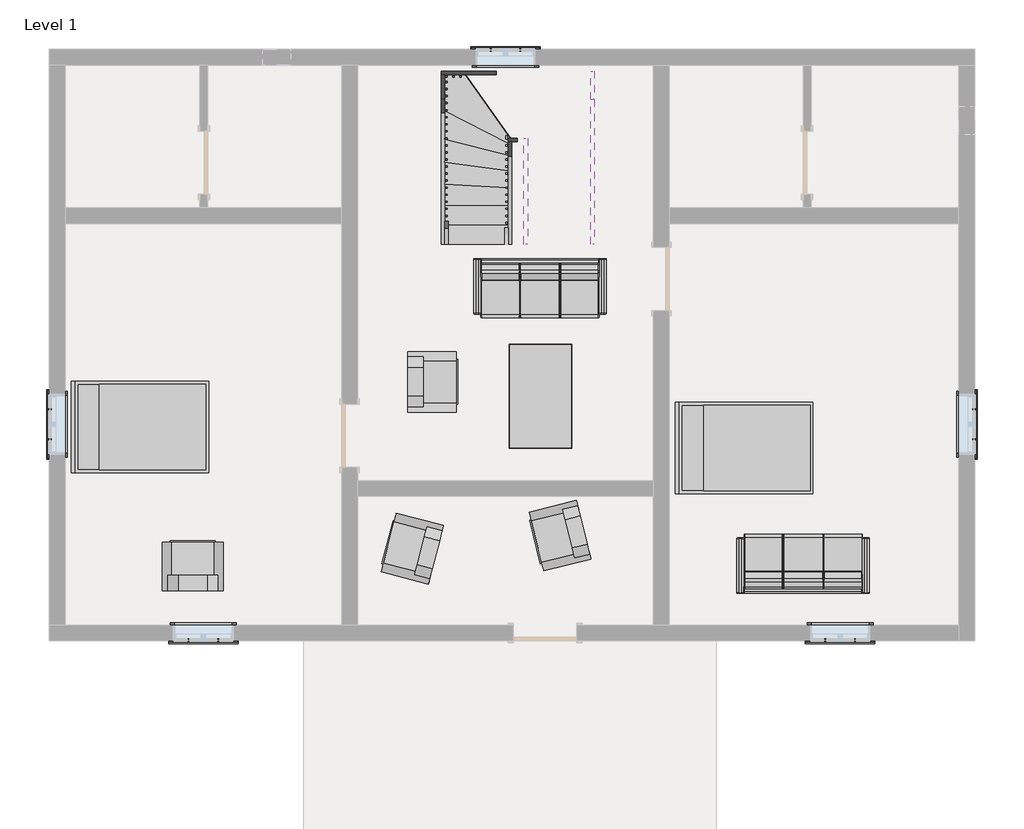
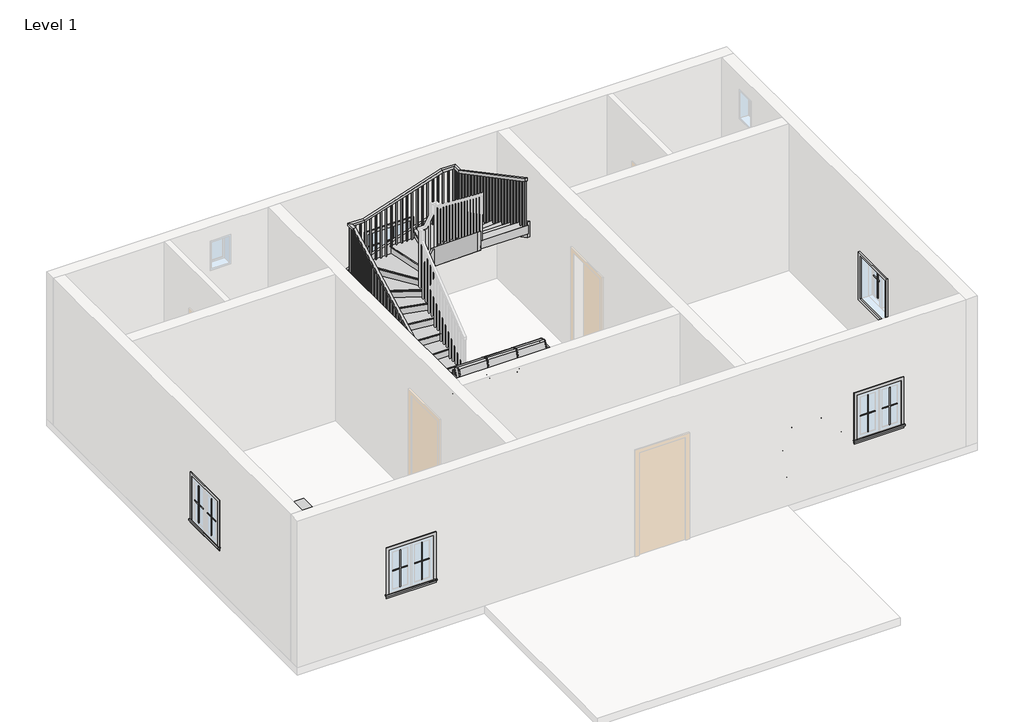
# One storey, part 2 of 2: 20 proxies, 9 furniture elements, 8 members, 1 railing, 1 stair flight.
"""IFC4 building model written with IfcOpenShell, lengths in millimetres."""

from ifc_helpers import new_model, si_unit, frame, origin, place, context, project, spatial, polyline, outline, extrude, faceted_brep, transform, mapped, element, save
from components import muntin_pattern_2x2_muntin_pattern_2x2_b3fe6957, muntin_pattern_2x2_muntin_pattern_2x2_3e0ecaf2, trim_window_exterior_flat_with_sill_41619996, trim_window_interior_flat_picture_frame_51c85655, furniture_2fc85b74, furniture_29a9adb8, furniture_57072a26, bed_17739_bed_17739_15c61121, chair_lounge_11461_couch_0866092f, dining_table_14755_dining_table_14755_d89cb775, stair_flight_9e59bd78

model = new_model("IFC4")

# Units and contexts
model_context = context("Model", 3, world=origin())
ifc_project = project(units=[si_unit("LENGTHUNIT", "METRE", prefix="MILLI")], contexts=[model_context])

# Site, building, storey
site = spatial("IfcSite", under=ifc_project)
building = spatial("IfcBuilding", under=site)
storey = spatial("IfcBuildingStorey", under=building, Name="Level 1", Elevation=0.0)

# Proxies
placement = place(None, origin())
muntin_pattern_2x2_muntin_pattern_2x2_shape = muntin_pattern_2x2_muntin_pattern_2x2_b3fe6957(model_context)
element("IfcBuildingElementProxy", 1, Name="Muntin Pattern_2x2 : Muntin Pattern_2x2", ObjectType="Muntin Pattern_2x2 : Muntin Pattern_2x2", at=placement, inside=storey, context=model_context, shape_type="MappedRepresentation", body=[
    mapped(muntin_pattern_2x2_muntin_pattern_2x2_shape, transform((-7325.4390964, 833.891032, 984.25), x_axis=(0.0, 1.0, 0.0), y_axis=(-1.0, 0.0, 0.0), z_axis=(0.0, 0.0, 1.0))),
])
element("IfcBuildingElementProxy", 2, Name="Muntin Pattern_2x2 : Muntin Pattern_2x2", ObjectType="Muntin Pattern_2x2 : Muntin Pattern_2x2", at=placement, inside=storey, context=model_context, shape_type="MappedRepresentation", body=[
    mapped(muntin_pattern_2x2_muntin_pattern_2x2_shape, transform((6006.3859036, 1262.516032, 984.25), x_axis=(0.0, -1.0, 0.0), y_axis=(1.0, 0.0, 0.0), z_axis=(0.0, 0.0, 1.0))),
])
element("IfcBuildingElementProxy", 3, Name="Muntin Pattern_2x2 : Muntin Pattern_2x2", ObjectType="Muntin Pattern_2x2 : Muntin Pattern_2x2", at=placement, inside=storey, context=model_context, shape_type="MappedRepresentation", body=[
    mapped(muntin_pattern_2x2_muntin_pattern_2x2_shape, transform((-967.5015964, 6448.878532, 984.25), x_axis=(1.0, 0.0, 0.0), y_axis=(0.0, 1.0, 0.0), z_axis=(0.0, 0.0, 1.0))),
])
element("IfcBuildingElementProxy", 4, Name="Muntin Pattern_2x2 : Muntin Pattern_2x2", ObjectType="Muntin Pattern_2x2 : Muntin Pattern_2x2", at=placement, inside=storey, context=model_context, shape_type="MappedRepresentation", body=[
    mapped(muntin_pattern_2x2_muntin_pattern_2x2_shape, transform((-4896.5640964, -2066.471468, 984.25), x_axis=(-1.0, 0.0, 0.0), y_axis=(0.0, -1.0, 0.0), z_axis=(0.0, 0.0, 1.0))),
])
element("IfcBuildingElementProxy", 5, Name="Muntin Pattern_2x2 : Muntin Pattern_2x2", ObjectType="Muntin Pattern_2x2 : Muntin Pattern_2x2", at=placement, inside=storey, context=model_context, shape_type="MappedRepresentation", body=[
    mapped(muntin_pattern_2x2_muntin_pattern_2x2_shape, transform((4287.1234036, -2066.471468, 984.25), x_axis=(-1.0, 0.0, 0.0), y_axis=(0.0, -1.0, 0.0), z_axis=(0.0, 0.0, 1.0))),
])
muntin_pattern_2x2_muntin_pattern_2x2_2_shape = muntin_pattern_2x2_muntin_pattern_2x2_3e0ecaf2(model_context)
element("IfcBuildingElementProxy", 6, Name="Muntin Pattern_2x2 : Muntin Pattern_2x2", ObjectType="Muntin Pattern_2x2 : Muntin Pattern_2x2", at=placement, inside=storey, context=model_context, shape_type="MappedRepresentation", body=[
    mapped(muntin_pattern_2x2_muntin_pattern_2x2_2_shape, transform((-7325.4390964, 1262.516032, 984.25), x_axis=(0.0, -1.0, 0.0), y_axis=(1.0, 0.0, 0.0), z_axis=(0.0, 0.0, 1.0))),
])
element("IfcBuildingElementProxy", 7, Name="Muntin Pattern_2x2 : Muntin Pattern_2x2", ObjectType="Muntin Pattern_2x2 : Muntin Pattern_2x2", at=placement, inside=storey, context=model_context, shape_type="MappedRepresentation", body=[
    mapped(muntin_pattern_2x2_muntin_pattern_2x2_2_shape, transform((6006.3859036, 833.891032, 984.25), x_axis=(0.0, 1.0, 0.0), y_axis=(-1.0, 0.0, 0.0), z_axis=(0.0, 0.0, 1.0))),
])
element("IfcBuildingElementProxy", 8, Name="Muntin Pattern_2x2 : Muntin Pattern_2x2", ObjectType="Muntin Pattern_2x2 : Muntin Pattern_2x2", at=placement, inside=storey, context=model_context, shape_type="MappedRepresentation", body=[
    mapped(muntin_pattern_2x2_muntin_pattern_2x2_2_shape, transform((-538.8765964, 6448.878532, 984.25), x_axis=(-1.0, 0.0, 0.0), y_axis=(0.0, -1.0, 0.0), z_axis=(0.0, 0.0, 1.0))),
])
element("IfcBuildingElementProxy", 9, Name="Muntin Pattern_2x2 : Muntin Pattern_2x2", ObjectType="Muntin Pattern_2x2 : Muntin Pattern_2x2", at=placement, inside=storey, context=model_context, shape_type="MappedRepresentation", body=[
    mapped(muntin_pattern_2x2_muntin_pattern_2x2_2_shape, transform((-5325.1890964, -2066.471468, 984.25), x_axis=(1.0, 0.0, 0.0), y_axis=(0.0, 1.0, 0.0), z_axis=(0.0, 0.0, 1.0))),
])
element("IfcBuildingElementProxy", 10, Name="Muntin Pattern_2x2 : Muntin Pattern_2x2", ObjectType="Muntin Pattern_2x2 : Muntin Pattern_2x2", at=placement, inside=storey, context=model_context, shape_type="MappedRepresentation", body=[
    mapped(muntin_pattern_2x2_muntin_pattern_2x2_2_shape, transform((3858.4984036, -2066.471468, 984.25), x_axis=(1.0, 0.0, 0.0), y_axis=(0.0, 1.0, 0.0), z_axis=(0.0, 0.0, 1.0))),
])
trim_window_exterior_flat_with_sill_shape = trim_window_exterior_flat_with_sill_41619996(model_context)
element("IfcBuildingElementProxy", 11, Name="Trim-Window-Exterior-Flat : with Sill", ObjectType="Trim-Window-Exterior-Flat : with Sill", at=placement, inside=storey, context=model_context, shape_type="MappedRepresentation", body=[
    mapped(trim_window_exterior_flat_with_sill_shape, transform((-7334.9640964, 1048.203532, 1828.8), x_axis=(0.0, -1.0, 0.0), y_axis=(0.0, 0.0, 1.0), z_axis=(-1.0, 0.0, 0.0))),
])
element("IfcBuildingElementProxy", 12, Name="Trim-Window-Exterior-Flat : with Sill", ObjectType="Trim-Window-Exterior-Flat : with Sill", at=placement, inside=storey, context=model_context, shape_type="MappedRepresentation", body=[
    mapped(trim_window_exterior_flat_with_sill_shape, transform((6015.9109036, 1048.203532, 1828.8), x_axis=(0.0, 1.0, 0.0), y_axis=(0.0, 0.0, 1.0), z_axis=(1.0, 0.0, 0.0))),
])
element("IfcBuildingElementProxy", 13, Name="Trim-Window-Exterior-Flat : with Sill", ObjectType="Trim-Window-Exterior-Flat : with Sill", at=placement, inside=storey, context=model_context, shape_type="MappedRepresentation", body=[
    mapped(trim_window_exterior_flat_with_sill_shape, transform((-753.1890964, 6458.403532, 1828.8), x_axis=(-1.0, 0.0, 0.0), y_axis=(0.0, 0.0, 1.0), z_axis=(0.0, 1.0, 0.0))),
])
element("IfcBuildingElementProxy", 14, Name="Trim-Window-Exterior-Flat : with Sill", ObjectType="Trim-Window-Exterior-Flat : with Sill", at=placement, inside=storey, context=model_context, shape_type="MappedRepresentation", body=[
    mapped(trim_window_exterior_flat_with_sill_shape, transform((-5110.8765964, -2075.996468, 1828.8), x_axis=(1.0, 0.0, 0.0), y_axis=(0.0, 0.0, 1.0), z_axis=(0.0, -1.0, 0.0))),
])
element("IfcBuildingElementProxy", 15, Name="Trim-Window-Exterior-Flat : with Sill", ObjectType="Trim-Window-Exterior-Flat : with Sill", at=placement, inside=storey, context=model_context, shape_type="MappedRepresentation", body=[
    mapped(trim_window_exterior_flat_with_sill_shape, transform((4072.8109036, -2075.996468, 1828.8), x_axis=(1.0, 0.0, 0.0), y_axis=(0.0, 0.0, 1.0), z_axis=(0.0, -1.0, 0.0))),
])
trim_window_interior_flat_picture_frame_shape = trim_window_interior_flat_picture_frame_51c85655(model_context)
element("IfcBuildingElementProxy", 16, Name="Trim-Window-Interior-Flat : Picture Frame", ObjectType="Trim-Window-Interior-Flat : Picture Frame", at=placement, inside=storey, context=model_context, shape_type="MappedRepresentation", body=[
    mapped(trim_window_interior_flat_picture_frame_shape, transform((-7106.3640964, 1048.203532, 1828.8), x_axis=(0.0, 1.0, 0.0), y_axis=(0.0, 0.0, 1.0), z_axis=(1.0, 0.0, 0.0))),
])
element("IfcBuildingElementProxy", 17, Name="Trim-Window-Interior-Flat : Picture Frame", ObjectType="Trim-Window-Interior-Flat : Picture Frame", at=placement, inside=storey, context=model_context, shape_type="MappedRepresentation", body=[
    mapped(trim_window_interior_flat_picture_frame_shape, transform((5787.3109036, 1048.203532, 1828.8), x_axis=(0.0, -1.0, 0.0), y_axis=(0.0, 0.0, 1.0), z_axis=(-1.0, 0.0, 0.0))),
])
element("IfcBuildingElementProxy", 18, Name="Trim-Window-Interior-Flat : Picture Frame", ObjectType="Trim-Window-Interior-Flat : Picture Frame", at=placement, inside=storey, context=model_context, shape_type="MappedRepresentation", body=[
    mapped(trim_window_interior_flat_picture_frame_shape, transform((-753.1890964, 6229.803532, 1828.8), x_axis=(1.0, 0.0, 0.0), y_axis=(0.0, 0.0, 1.0), z_axis=(0.0, -1.0, 0.0))),
])
element("IfcBuildingElementProxy", 19, Name="Trim-Window-Interior-Flat : Picture Frame", ObjectType="Trim-Window-Interior-Flat : Picture Frame", at=placement, inside=storey, context=model_context, shape_type="MappedRepresentation", body=[
    mapped(trim_window_interior_flat_picture_frame_shape, transform((-5110.8765964, -1847.396468, 1828.8), x_axis=(-1.0, 0.0, 0.0), y_axis=(0.0, 0.0, 1.0), z_axis=(0.0, 1.0, 0.0))),
])
element("IfcBuildingElementProxy", 20, Name="Trim-Window-Interior-Flat : Picture Frame", ObjectType="Trim-Window-Interior-Flat : Picture Frame", at=placement, inside=storey, context=model_context, shape_type="MappedRepresentation", body=[
    mapped(trim_window_interior_flat_picture_frame_shape, transform((4072.8109036, -1847.396468, 1828.8), x_axis=(-1.0, 0.0, 0.0), y_axis=(0.0, 0.0, 1.0), z_axis=(0.0, 1.0, 0.0))),
])

# Furniture
furniture_shape = furniture_2fc85b74(model_context)
furniture_2_shape = furniture_29a9adb8(model_context)
furniture_3_shape = furniture_57072a26(model_context)
element("IfcFurniture", 21, at=placement, inside=storey, context=model_context, shape_type="MappedRepresentation", body=[
    mapped(furniture_shape, transform((-255.3775912, 2638.3556028, 0.0), x_axis=(1.0, 0.0, 0.0), y_axis=(0.0, 1.0, 0.0), z_axis=(0.0, 0.0, 1.0))),
    mapped(furniture_2_shape, transform((-255.3775912, 2638.3556028, 0.0), x_axis=(1.0, 0.0, 0.0), y_axis=(0.0, 1.0, 0.0), z_axis=(0.0, 0.0, 1.0))),
    mapped(furniture_3_shape, transform((-255.3775912, 2638.3556028, 0.0), x_axis=(1.0, 0.0, 0.0), y_axis=(0.0, 1.0, 0.0), z_axis=(0.0, 0.0, 1.0))),
])
element("IfcFurniture", 22, at=placement, inside=storey, context=model_context, shape_type="MappedRepresentation", body=[
    mapped(furniture_shape, transform((3539.4109036, -590.096468, 0.0), x_axis=(-1.0, 0.0, 0.0), y_axis=(0.0, -1.0, 0.0), z_axis=(0.0, 0.0, 1.0))),
    mapped(furniture_2_shape, transform((3539.4109036, -590.096468, 0.0), x_axis=(-1.0, 0.0, 0.0), y_axis=(0.0, -1.0, 0.0), z_axis=(0.0, 0.0, 1.0))),
    mapped(furniture_3_shape, transform((3539.4109036, -590.096468, 0.0), x_axis=(-1.0, 0.0, 0.0), y_axis=(0.0, -1.0, 0.0), z_axis=(0.0, 0.0, 1.0))),
])
bed_17739_bed_17739_shape = bed_17739_bed_17739_15c61121(model_context)
element("IfcFurniture", 23, ObjectType="Bed_17739 : Bed_17739", at=placement, inside=storey, context=model_context, shape_type="MappedRepresentation", body=[
    mapped(bed_17739_bed_17739_shape, transform((-6001.4640964, 1010.103532, 0.0), x_axis=(0.0, 1.0, 0.0), y_axis=(-1.0, 0.0, 0.0), z_axis=(0.0, 0.0, 1.0))),
])
element("IfcFurniture", 24, ObjectType="Bed_17739 : Bed_17739", at=placement, inside=storey, context=model_context, shape_type="MappedRepresentation", body=[
    mapped(bed_17739_bed_17739_shape, transform((2713.9109036, 705.303532, 0.0), x_axis=(0.0, 1.0, 0.0), y_axis=(-1.0, 0.0, 0.0), z_axis=(0.0, 0.0, 1.0))),
])
chair_lounge_11461_couch_shape = chair_lounge_11461_couch_0866092f(model_context)
element("IfcFurniture", 25, ObjectType="Chair-Lounge_11461 : Couch", at=placement, inside=storey, context=model_context, shape_type="MappedRepresentation", body=[
    mapped(chair_lounge_11461_couch_shape, transform((-5264.5951021, -1353.5250534, 0.0), x_axis=(-1.0, 0.0, 0.0), y_axis=(0.0, -1.0, 0.0), z_axis=(0.0, 0.0, 1.0))),
])
element("IfcFurniture", 26, ObjectType="Chair-Lounge_11461 : Couch", at=placement, inside=storey, context=model_context, shape_type="MappedRepresentation", body=[
    mapped(chair_lounge_11461_couch_shape, transform((-2164.5215733, 1660.4831648, 0.0), x_axis=(0.0, 1.0, 0.0), y_axis=(-1.0, 0.0, 0.0), z_axis=(0.0, 0.0, 1.0))),
])
element("IfcFurniture", 27, ObjectType="Chair-Lounge_11461 : Couch", at=placement, inside=storey, context=model_context, shape_type="MappedRepresentation", body=[
    mapped(chair_lounge_11461_couch_shape, transform((-1757.4278992, -832.4672327, 0.0), x_axis=(-0.25020656802293967, -0.9681924774125144, 0.0), y_axis=(0.9681924774125144, -0.25020656802293967, 0.0), z_axis=(0.0, 0.0, 1.0))),
])
element("IfcFurniture", 28, ObjectType="Chair-Lounge_11461 : Couch", at=placement, inside=storey, context=model_context, shape_type="MappedRepresentation", body=[
    mapped(chair_lounge_11461_couch_shape, transform((374.96053, -475.589841, 0.0), x_axis=(0.23930720047404658, -0.9709439035295884, 0.0), y_axis=(0.9709439035295884, 0.23930720047404658, 0.0), z_axis=(0.0, 0.0, 1.0))),
])
dining_table_14755_dining_table_14755_shape = dining_table_14755_dining_table_14755_d89cb775(model_context)
element("IfcFurniture", 29, ObjectType="Dining_table_14755 : Dining_table_14755", at=placement, inside=storey, context=model_context, shape_type="MappedRepresentation", body=[
    mapped(dining_table_14755_dining_table_14755_shape, transform((199.3109036, 705.303532, 0.0), x_axis=(0.0, 1.0, 0.0), y_axis=(-1.0, 0.0, 0.0), z_axis=(0.0, 0.0, 1.0))),
])

# Members
element("IfcMember", 30, ObjectType="Stringer - 2\" Width", at=placement, inside=storey, context=model_context, shape_type="SweptSolid", body=[
    extrude(outline(polyline([(3647.9718401, 0.0), (3647.9718401, 229.639954), (5735.3890318, 1305.3956453), (5735.3890318, 962.500629), (3867.7341577, 0.0), (3647.9718401, 0.0)])), frame((-1680.2890964, 0.0, 0.0), z_axis=(1.0, 0.0, 0.0), x_axis=(0.0, 1.0, 0.0)), (0.0, 0.0, 1.0), 50.8),
])
element("IfcMember", 31, ObjectType="Stringer - 2\" Width", at=placement, inside=storey, context=model_context, shape_type="SweptSolid", body=[
    extrude(outline(polyline([(-1629.4890964, 5735.3890318), (-1680.2890964, 5735.3890318), (-1680.2890964, 6090.103532), (-1629.4890964, 6090.103532), (-1629.4890964, 5735.3890318)])), frame((0.0, 0.0, 962.500629), z_axis=(0.0, 0.0, 1.0), x_axis=(1.0, 0.0, 0.0)), (0.0, 0.0, 1.0), 342.8950162),
])
element("IfcMember", 32, ObjectType="Stringer - 2\" Width", at=placement, inside=storey, context=model_context, shape_type="SweptSolid", body=[
    extrude(outline(polyline([(1289.0952212, -1680.2890964), (1000.5956453, -1680.2890964), (1000.5956453, -1510.7666134), (1638.9682298, 478.7109036), (1969.9972697, 478.7109036), (1969.9972697, 441.7307863), (1289.0952212, -1680.2890964)])), frame((0.0, 6090.103532, 0.0), z_axis=(0.0, 1.0, 0.0), x_axis=(0.0, 0.0, 1.0)), (0.0, 0.0, 1.0), 50.8),
])
element("IfcMember", 33, ObjectType="Stringer - 2\" Width", at=placement, inside=storey, context=model_context, shape_type="SweptSolid", body=[
    extrude(outline(polyline([(478.7109036, 6140.903532), (529.5109036, 6140.903532), (529.5109036, 5735.3890318), (478.7109036, 5735.3890318), (478.7109036, 6140.903532)])), frame((0.0, 0.0, 1649.8904473), z_axis=(0.0, 0.0, 1.0), x_axis=(1.0, 0.0, 0.0)), (0.0, 0.0, 1.0), 320.1068224),
])
element("IfcMember", 34, ObjectType="Stringer - 2\" Width", at=placement, inside=storey, context=model_context, shape_type="SweptSolid", body=[
    extrude(outline(polyline([(5735.3890318, 1969.9972697), (5735.3890318, 1649.8904473), (3647.9718401, 2725.6461385), (3647.9718401, 3045.7529609), (5735.3890318, 1969.9972697)])), frame((478.7109036, 0.0, 0.0), z_axis=(1.0, 0.0, 0.0), x_axis=(0.0, 1.0, 0.0)), (0.0, 0.0, 1.0), 50.8),
])
element("IfcMember", 35, ObjectType="Stringer - 2\" Width", at=placement, inside=storey, context=model_context, shape_type="SweptSolid", body=[
    extrude(outline(polyline([(3647.9718401, 0.0), (3647.9718401, 176.1764461), (5124.903532, 1380.418648), (5124.903532, 987.1410923), (3914.2334847, 0.0), (3647.9718401, 0.0)])), frame((-715.0890964, 0.0, 0.0), z_axis=(1.0, 0.0, 0.0), x_axis=(0.0, 1.0, 0.0)), (0.0, 0.0, 1.0), 50.8),
])
element("IfcMember", 36, ObjectType="Stringer - 2\" Width", at=placement, inside=storey, context=model_context, shape_type="SweptSolid", body=[
    extrude(outline(polyline([(1573.2682978, -715.0890964), (1028.5617647, -715.0890964), (1028.5617647, -680.846879), (1360.465107, -486.4890964), (1926.1409689, -486.4890964), (1926.1409689, -508.4519789), (1573.2682978, -715.0890964)])), frame((0.0, 5124.903532, 0.0), z_axis=(0.0, 1.0, 0.0), x_axis=(0.0, 0.0, 1.0)), (0.0, 0.0, 1.0), 50.8),
])
element("IfcMember", 37, ObjectType="Stringer - 2\" Width", at=placement, inside=storey, context=model_context, shape_type="SweptSolid", body=[
    extrude(outline(polyline([(5175.703532, 1926.1409689), (5175.703532, 1532.8634131), (3647.9718401, 2778.5262875), (3647.9718401, 3171.8038432), (5175.703532, 1926.1409689)])), frame((-486.4890964, 0.0, 0.0), z_axis=(1.0, 0.0, 0.0), x_axis=(0.0, 1.0, 0.0)), (0.0, 0.0, 1.0), 50.8),
])

# Railing
element("IfcRailing", 38, ObjectType="Handrail - Rectangular", at=placement, inside=storey, context=model_context, shape_type="SolidModel", body=[
    faceted_brep([(-1629.4890964, 3647.9718401, 1083.7333333), (-1629.4890964, 3647.9718401, 1026.2742652), (-1578.6890964, 3647.9718401, 1026.2742652), (-1578.6890964, 3647.9718401, 1083.7333333), (-1629.4890964, 5905.6969022, 2277.0239201), (-1629.4890964, 5918.2959667, 2226.2239201), (-1578.6890964, 5918.2959667, 2226.2239201), (-1578.6890964, 5905.6969022, 2277.0239201), (-1629.4890964, 6090.103532, 2277.0239201), (-1629.4890964, 6090.103532, 2226.2239201), (-1578.6890964, 6039.303532, 2226.2239201), (-1578.6890964, 6039.303532, 2277.0239201), (-1342.1772142, 6090.103532, 2277.0239201), (-1334.2266381, 6090.103532, 2226.2239201), (-1334.2266381, 6039.303532, 2226.2239201), (-1342.1772142, 6039.303532, 2277.0239201), (191.3990215, 6090.103532, 2769.1094132), (199.3495976, 6090.103532, 2718.3094132), (199.3495976, 6039.303532, 2718.3094132), (191.3990215, 6039.303532, 2769.1094132), (478.7109036, 6090.103532, 2769.1094132), (478.7109036, 6090.103532, 2718.3094132), (427.9109036, 6039.303532, 2718.3094132), (427.9109036, 6039.303532, 2769.1094132), (478.7109036, 5905.6969022, 2769.1094132), (478.7109036, 5893.0978376, 2718.3094132), (427.9109036, 5893.0978376, 2718.3094132), (427.9109036, 5905.6969022, 2769.1094132), (478.7109036, 3647.9718401, 3962.4), (427.9109036, 3647.9718401, 3962.4), (427.9109036, 3647.9718401, 3904.9409318), (478.7109036, 3647.9718401, 3904.9409318)], [[[0, 1, 2, 3]], [[1, 0, 4, 5]], [[2, 1, 5, 6]], [[3, 2, 6, 7]], [[0, 3, 7, 4]], [[5, 4, 8, 9]], [[6, 5, 9, 10]], [[7, 6, 10, 11]], [[4, 7, 11, 8]], [[9, 8, 12, 13]], [[10, 9, 13, 14]], [[11, 10, 14, 15]], [[8, 11, 15, 12]], [[13, 12, 16, 17]], [[14, 13, 17, 18]], [[15, 14, 18, 19]], [[12, 15, 19, 16]], [[17, 16, 20, 21]], [[18, 17, 21, 22]], [[19, 18, 22, 23]], [[16, 19, 23, 20]], [[21, 20, 24, 25]], [[22, 21, 25, 26]], [[23, 22, 26, 27]], [[20, 23, 27, 24]], [[28, 29, 30, 31]], [[25, 24, 28, 31]], [[26, 25, 31, 30]], [[27, 26, 30, 29]], [[24, 27, 29, 28]]]),
    extrude(outline(polyline([(3737.428532, 3857.6597858), (3737.428532, 2878.6666667), (3718.378532, 2878.6666667), (3718.378532, 3867.7284102), (3737.428532, 3857.6597858)])), frame((443.7859036, 0.0, 0.0), z_axis=(1.0, 0.0, 0.0), x_axis=(0.0, 1.0, 0.0)), (0.0, 0.0, 1.0), 19.05),
    extrude(outline(polyline([(3839.028532, 3803.9604556), (3839.028532, 2878.6666667), (3819.978532, 2878.6666667), (3819.978532, 3814.02908), (3839.028532, 3803.9604556)])), frame((443.7859036, 0.0, 0.0), z_axis=(1.0, 0.0, 0.0), x_axis=(0.0, 1.0, 0.0)), (0.0, 0.0, 1.0), 19.05),
    extrude(outline(polyline([(3940.628532, 3750.2611254), (3940.628532, 2709.3333333), (3921.578532, 2709.3333333), (3921.578532, 3760.3297498), (3940.628532, 3750.2611254)])), frame((443.7859036, 0.0, 0.0), z_axis=(1.0, 0.0, 0.0), x_axis=(0.0, 1.0, 0.0)), (0.0, 0.0, 1.0), 19.05),
    extrude(outline(polyline([(4042.228532, 3696.5617952), (4042.228532, 2709.3333333), (4023.178532, 2709.3333333), (4023.178532, 3706.6304196), (4042.228532, 3696.5617952)])), frame((443.7859036, 0.0, 0.0), z_axis=(1.0, 0.0, 0.0), x_axis=(0.0, 1.0, 0.0)), (0.0, 0.0, 1.0), 19.05),
    extrude(outline(polyline([(4143.828532, 3642.862465), (4143.828532, 2709.3333333), (4124.778532, 2709.3333333), (4124.778532, 3652.9310894), (4143.828532, 3642.862465)])), frame((443.7859036, 0.0, 0.0), z_axis=(1.0, 0.0, 0.0), x_axis=(0.0, 1.0, 0.0)), (0.0, 0.0, 1.0), 19.05),
    extrude(outline(polyline([(4245.428532, 3589.1631348), (4245.428532, 2540.0), (4226.378532, 2540.0), (4226.378532, 3599.2317592), (4245.428532, 3589.1631348)])), frame((443.7859036, 0.0, 0.0), z_axis=(1.0, 0.0, 0.0), x_axis=(0.0, 1.0, 0.0)), (0.0, 0.0, 1.0), 19.05),
    extrude(outline(polyline([(4347.028532, 3535.4638046), (4347.028532, 2540.0), (4327.978532, 2540.0), (4327.978532, 3545.532429), (4347.028532, 3535.4638046)])), frame((443.7859036, 0.0, 0.0), z_axis=(1.0, 0.0, 0.0), x_axis=(0.0, 1.0, 0.0)), (0.0, 0.0, 1.0), 19.05),
    extrude(outline(polyline([(4448.628532, 3481.7644744), (4448.628532, 2540.0), (4429.578532, 2540.0), (4429.578532, 3491.8330988), (4448.628532, 3481.7644744)])), frame((443.7859036, 0.0, 0.0), z_axis=(1.0, 0.0, 0.0), x_axis=(0.0, 1.0, 0.0)), (0.0, 0.0, 1.0), 19.05),
    extrude(outline(polyline([(4550.228532, 3428.0651442), (4550.228532, 2370.6666667), (4531.178532, 2370.6666667), (4531.178532, 3438.1337686), (4550.228532, 3428.0651442)])), frame((443.7859036, 0.0, 0.0), z_axis=(1.0, 0.0, 0.0), x_axis=(0.0, 1.0, 0.0)), (0.0, 0.0, 1.0), 19.05),
    extrude(outline(polyline([(4651.828532, 3374.365814), (4651.828532, 2370.6666667), (4632.778532, 2370.6666667), (4632.778532, 3384.4344384), (4651.828532, 3374.365814)])), frame((443.7859036, 0.0, 0.0), z_axis=(1.0, 0.0, 0.0), x_axis=(0.0, 1.0, 0.0)), (0.0, 0.0, 1.0), 19.05),
    extrude(outline(polyline([(4753.428532, 3320.6664838), (4753.428532, 2370.6666667), (4734.378532, 2370.6666667), (4734.378532, 3330.7351082), (4753.428532, 3320.6664838)])), frame((443.7859036, 0.0, 0.0), z_axis=(1.0, 0.0, 0.0), x_axis=(0.0, 1.0, 0.0)), (0.0, 0.0, 1.0), 19.05),
    extrude(outline(polyline([(4855.028532, 3266.9671536), (4855.028532, 2201.3333333), (4835.978532, 2201.3333333), (4835.978532, 3277.035778), (4855.028532, 3266.9671536)])), frame((443.7859036, 0.0, 0.0), z_axis=(1.0, 0.0, 0.0), x_axis=(0.0, 1.0, 0.0)), (0.0, 0.0, 1.0), 19.05),
    extrude(outline(polyline([(4956.628532, 3213.2678234), (4956.628532, 2201.3333333), (4937.578532, 2201.3333333), (4937.578532, 3223.3364478), (4956.628532, 3213.2678234)])), frame((443.7859036, 0.0, 0.0), z_axis=(1.0, 0.0, 0.0), x_axis=(0.0, 1.0, 0.0)), (0.0, 0.0, 1.0), 19.05),
    extrude(outline(polyline([(5058.228532, 3159.5684932), (5058.228532, 2201.3333333), (5039.178532, 2201.3333333), (5039.178532, 3169.6371176), (5058.228532, 3159.5684932)])), frame((443.7859036, 0.0, 0.0), z_axis=(1.0, 0.0, 0.0), x_axis=(0.0, 1.0, 0.0)), (0.0, 0.0, 1.0), 19.05),
    extrude(outline(polyline([(5159.828532, 3105.869163), (5159.828532, 2201.3333333), (5140.778532, 2201.3333333), (5140.778532, 3115.9377874), (5159.828532, 3105.869163)])), frame((443.7859036, 0.0, 0.0), z_axis=(1.0, 0.0, 0.0), x_axis=(0.0, 1.0, 0.0)), (0.0, 0.0, 1.0), 19.05),
    extrude(outline(polyline([(5261.428532, 3052.1698328), (5261.428532, 2032.0), (5242.378532, 2032.0), (5242.378532, 3062.2384572), (5261.428532, 3052.1698328)])), frame((443.7859036, 0.0, 0.0), z_axis=(1.0, 0.0, 0.0), x_axis=(0.0, 1.0, 0.0)), (0.0, 0.0, 1.0), 19.05),
    extrude(outline(polyline([(5363.028532, 2998.4705026), (5363.028532, 2032.0), (5343.978532, 2032.0), (5343.978532, 3008.539127), (5363.028532, 2998.4705026)])), frame((443.7859036, 0.0, 0.0), z_axis=(1.0, 0.0, 0.0), x_axis=(0.0, 1.0, 0.0)), (0.0, 0.0, 1.0), 19.05),
    extrude(outline(polyline([(5464.628532, 2944.7711724), (5464.628532, 2032.0), (5445.578532, 2032.0), (5445.578532, 2954.8397968), (5464.628532, 2944.7711724)])), frame((443.7859036, 0.0, 0.0), z_axis=(1.0, 0.0, 0.0), x_axis=(0.0, 1.0, 0.0)), (0.0, 0.0, 1.0), 19.05),
    extrude(outline(polyline([(5566.228532, 2891.0718422), (5566.228532, 2032.0), (5547.178532, 2032.0), (5547.178532, 2901.1404666), (5566.228532, 2891.0718422)])), frame((443.7859036, 0.0, 0.0), z_axis=(1.0, 0.0, 0.0), x_axis=(0.0, 1.0, 0.0)), (0.0, 0.0, 1.0), 19.05),
    extrude(outline(polyline([(5667.828532, 2837.372512), (5667.828532, 1862.6666667), (5648.778532, 1862.6666667), (5648.778532, 2847.4411364), (5667.828532, 2837.372512)])), frame((443.7859036, 0.0, 0.0), z_axis=(1.0, 0.0, 0.0), x_axis=(0.0, 1.0, 0.0)), (0.0, 0.0, 1.0), 19.05),
    extrude(outline(polyline([(5769.428532, 2783.6731818), (5769.428532, 1862.6666667), (5750.378532, 1862.6666667), (5750.378532, 2793.7418062), (5769.428532, 2783.6731818)])), frame((443.7859036, 0.0, 0.0), z_axis=(1.0, 0.0, 0.0), x_axis=(0.0, 1.0, 0.0)), (0.0, 0.0, 1.0), 19.05),
    extrude(outline(polyline([(5871.028532, 2729.9738516), (5871.028532, 1862.6666667), (5851.978532, 1862.6666667), (5851.978532, 2740.042476), (5871.028532, 2729.9738516)])), frame((443.7859036, 0.0, 0.0), z_axis=(1.0, 0.0, 0.0), x_axis=(0.0, 1.0, 0.0)), (0.0, 0.0, 1.0), 19.05),
    extrude(outline(polyline([(462.8359036, 5972.628532), (462.8359036, 5953.578532), (443.7859036, 5953.578532), (443.7859036, 5972.628532), (462.8359036, 5972.628532)])), frame((0.0, 0.0, 1862.6666667), z_axis=(0.0, 0.0, 1.0), x_axis=(1.0, 0.0, 0.0)), (0.0, 0.0, 1.0), 855.6427466),
    extrude(outline(polyline([(418.3859036, 6074.228532), (437.4359036, 6074.228532), (437.4359036, 6055.178532), (418.3859036, 6055.178532), (418.3859036, 6074.228532)])), frame((0.0, 0.0, 1862.6666667), z_axis=(0.0, 0.0, 1.0), x_axis=(1.0, 0.0, 0.0)), (0.0, 0.0, 1.0), 855.6427466),
    extrude(outline(polyline([(316.7859036, 6074.228532), (335.8359036, 6074.228532), (335.8359036, 6055.178532), (316.7859036, 6055.178532), (316.7859036, 6074.228532)])), frame((0.0, 0.0, 1862.6666667), z_axis=(0.0, 0.0, 1.0), x_axis=(1.0, 0.0, 0.0)), (0.0, 0.0, 1.0), 855.6427466),
    extrude(outline(polyline([(215.1859036, 6074.228532), (234.2359036, 6074.228532), (234.2359036, 6055.178532), (215.1859036, 6055.178532), (215.1859036, 6074.228532)])), frame((0.0, 0.0, 1862.6666667), z_axis=(0.0, 0.0, 1.0), x_axis=(1.0, 0.0, 0.0)), (0.0, 0.0, 1.0), 855.6427466),
    extrude(outline(polyline([(2690.7900316, 113.5859036), (1693.3333333, 113.5859036), (1693.3333333, 132.6359036), (2696.9026907, 132.6359036), (2690.7900316, 113.5859036)])), frame((0.0, 6055.178532, 0.0), z_axis=(0.0, 1.0, 0.0), x_axis=(0.0, 0.0, 1.0)), (0.0, 0.0, 1.0), 19.05),
    extrude(outline(polyline([(2658.1891834, 11.9859036), (1693.3333333, 11.9859036), (1693.3333333, 31.0359036), (2664.3018425, 31.0359036), (2658.1891834, 11.9859036)])), frame((0.0, 6055.178532, 0.0), z_axis=(0.0, 1.0, 0.0), x_axis=(0.0, 0.0, 1.0)), (0.0, 0.0, 1.0), 19.05),
    extrude(outline(polyline([(2625.5883352, -89.6140964), (1693.3333333, -89.6140964), (1693.3333333, -70.5640964), (2631.7009942, -70.5640964), (2625.5883352, -89.6140964)])), frame((0.0, 6055.178532, 0.0), z_axis=(0.0, 1.0, 0.0), x_axis=(0.0, 0.0, 1.0)), (0.0, 0.0, 1.0), 19.05),
    extrude(outline(polyline([(2592.987487, -191.2140964), (1693.3333333, -191.2140964), (1693.3333333, -172.1640964), (2599.100146, -172.1640964), (2592.987487, -191.2140964)])), frame((0.0, 6055.178532, 0.0), z_axis=(0.0, 1.0, 0.0), x_axis=(0.0, 0.0, 1.0)), (0.0, 0.0, 1.0), 19.05),
    extrude(outline(polyline([(2560.3866387, -292.8140964), (1693.3333333, -292.8140964), (1693.3333333, -273.7640964), (2566.4992978, -273.7640964), (2560.3866387, -292.8140964)])), frame((0.0, 6055.178532, 0.0), z_axis=(0.0, 1.0, 0.0), x_axis=(0.0, 0.0, 1.0)), (0.0, 0.0, 1.0), 19.05),
    extrude(outline(polyline([(2527.7857905, -394.4140964), (1524.0, -394.4140964), (1524.0, -375.3640964), (2533.8984495, -375.3640964), (2527.7857905, -394.4140964)])), frame((0.0, 6055.178532, 0.0), z_axis=(0.0, 1.0, 0.0), x_axis=(0.0, 0.0, 1.0)), (0.0, 0.0, 1.0), 19.05),
    extrude(outline(polyline([(2495.1849423, -496.0140964), (1524.0, -496.0140964), (1524.0, -476.9640964), (2501.2976013, -476.9640964), (2495.1849423, -496.0140964)])), frame((0.0, 6055.178532, 0.0), z_axis=(0.0, 1.0, 0.0), x_axis=(0.0, 0.0, 1.0)), (0.0, 0.0, 1.0), 19.05),
    extrude(outline(polyline([(2462.5840941, -597.6140964), (1524.0, -597.6140964), (1524.0, -578.5640964), (2468.6967531, -578.5640964), (2462.5840941, -597.6140964)])), frame((0.0, 6055.178532, 0.0), z_axis=(0.0, 1.0, 0.0), x_axis=(0.0, 0.0, 1.0)), (0.0, 0.0, 1.0), 19.05),
    extrude(outline(polyline([(2429.9832458, -699.2140964), (1524.0, -699.2140964), (1524.0, -680.1640964), (2436.0959049, -680.1640964), (2429.9832458, -699.2140964)])), frame((0.0, 6055.178532, 0.0), z_axis=(0.0, 1.0, 0.0), x_axis=(0.0, 0.0, 1.0)), (0.0, 0.0, 1.0), 19.05),
    extrude(outline(polyline([(2397.3823976, -800.8140964), (1524.0, -800.8140964), (1524.0, -781.7640964), (2403.4950566, -781.7640964), (2397.3823976, -800.8140964)])), frame((0.0, 6055.178532, 0.0), z_axis=(0.0, 1.0, 0.0), x_axis=(0.0, 0.0, 1.0)), (0.0, 0.0, 1.0), 19.05),
    extrude(outline(polyline([(2364.7815494, -902.4140964), (1354.6666667, -902.4140964), (1354.6666667, -883.3640964), (2370.8942084, -883.3640964), (2364.7815494, -902.4140964)])), frame((0.0, 6055.178532, 0.0), z_axis=(0.0, 1.0, 0.0), x_axis=(0.0, 0.0, 1.0)), (0.0, 0.0, 1.0), 19.05),
    extrude(outline(polyline([(2332.1807011, -1004.0140964), (1354.6666667, -1004.0140964), (1354.6666667, -984.9640964), (2338.2933602, -984.9640964), (2332.1807011, -1004.0140964)])), frame((0.0, 6055.178532, 0.0), z_axis=(0.0, 1.0, 0.0), x_axis=(0.0, 0.0, 1.0)), (0.0, 0.0, 1.0), 19.05),
    extrude(outline(polyline([(2299.5798529, -1105.6140964), (1354.6666667, -1105.6140964), (1354.6666667, -1086.5640964), (2305.692512, -1086.5640964), (2299.5798529, -1105.6140964)])), frame((0.0, 6055.178532, 0.0), z_axis=(0.0, 1.0, 0.0), x_axis=(0.0, 0.0, 1.0)), (0.0, 0.0, 1.0), 19.05),
    extrude(outline(polyline([(2266.9790047, -1207.2140964), (1354.6666667, -1207.2140964), (1354.6666667, -1188.1640964), (2273.0916637, -1188.1640964), (2266.9790047, -1207.2140964)])), frame((0.0, 6055.178532, 0.0), z_axis=(0.0, 1.0, 0.0), x_axis=(0.0, 0.0, 1.0)), (0.0, 0.0, 1.0), 19.05),
    extrude(outline(polyline([(2234.3781565, -1308.8140964), (1354.6666667, -1308.8140964), (1354.6666667, -1289.7640964), (2240.4908155, -1289.7640964), (2234.3781565, -1308.8140964)])), frame((0.0, 6055.178532, 0.0), z_axis=(0.0, 1.0, 0.0), x_axis=(0.0, 0.0, 1.0)), (0.0, 0.0, 1.0), 19.05),
    extrude(outline(polyline([(-1410.4140964, 6074.228532), (-1391.3640964, 6074.228532), (-1391.3640964, 6055.178532), (-1410.4140964, 6055.178532), (-1410.4140964, 6074.228532)])), frame((0.0, 0.0, 1185.3333333), z_axis=(0.0, 0.0, 1.0), x_axis=(1.0, 0.0, 0.0)), (0.0, 0.0, 1.0), 1040.8905868),
    extrude(outline(polyline([(-1512.0140964, 6074.228532), (-1492.9640964, 6074.228532), (-1492.9640964, 6055.178532), (-1512.0140964, 6055.178532), (-1512.0140964, 6074.228532)])), frame((0.0, 0.0, 1185.3333333), z_axis=(0.0, 0.0, 1.0), x_axis=(1.0, 0.0, 0.0)), (0.0, 0.0, 1.0), 1040.8905868),
    extrude(outline(polyline([(-1613.6140964, 5975.2468401), (-1613.6140964, 5994.2968401), (-1594.5640964, 5994.2968401), (-1594.5640964, 5975.2468401), (-1613.6140964, 5975.2468401)])), frame((0.0, 0.0, 1185.3333333), z_axis=(0.0, 0.0, 1.0), x_axis=(1.0, 0.0, 0.0)), (0.0, 0.0, 1.0), 1040.8905868),
    extrude(outline(polyline([(5892.6968401, 2212.6938418), (5892.6968401, 1185.3333333), (5873.6468401, 1185.3333333), (5873.6468401, 2202.6252174), (5892.6968401, 2212.6938418)])), frame((-1613.6140964, 0.0, 0.0), z_axis=(1.0, 0.0, 0.0), x_axis=(0.0, 1.0, 0.0)), (0.0, 0.0, 1.0), 19.05),
    extrude(outline(polyline([(5791.0968401, 2158.9945116), (5791.0968401, 1185.3333333), (5772.0468401, 1185.3333333), (5772.0468401, 2148.9258872), (5791.0968401, 2158.9945116)])), frame((-1613.6140964, 0.0, 0.0), z_axis=(1.0, 0.0, 0.0), x_axis=(0.0, 1.0, 0.0)), (0.0, 0.0, 1.0), 19.05),
    extrude(outline(polyline([(5689.4968401, 2105.2951814), (5689.4968401, 1185.3333333), (5670.4468401, 1185.3333333), (5670.4468401, 2095.226557), (5689.4968401, 2105.2951814)])), frame((-1613.6140964, 0.0, 0.0), z_axis=(1.0, 0.0, 0.0), x_axis=(0.0, 1.0, 0.0)), (0.0, 0.0, 1.0), 19.05),
    extrude(outline(polyline([(5587.8968401, 2051.5958512), (5587.8968401, 1185.3333333), (5568.8468401, 1185.3333333), (5568.8468401, 2041.5272268), (5587.8968401, 2051.5958512)])), frame((-1613.6140964, 0.0, 0.0), z_axis=(1.0, 0.0, 0.0), x_axis=(0.0, 1.0, 0.0)), (0.0, 0.0, 1.0), 19.05),
    extrude(outline(polyline([(5486.2968401, 1997.896521), (5486.2968401, 1016.0), (5467.2468401, 1016.0), (5467.2468401, 1987.8278966), (5486.2968401, 1997.896521)])), frame((-1613.6140964, 0.0, 0.0), z_axis=(1.0, 0.0, 0.0), x_axis=(0.0, 1.0, 0.0)), (0.0, 0.0, 1.0), 19.05),
    extrude(outline(polyline([(5384.6968401, 1944.1971908), (5384.6968401, 1016.0), (5365.6468401, 1016.0), (5365.6468401, 1934.1285664), (5384.6968401, 1944.1971908)])), frame((-1613.6140964, 0.0, 0.0), z_axis=(1.0, 0.0, 0.0), x_axis=(0.0, 1.0, 0.0)), (0.0, 0.0, 1.0), 19.05),
    extrude(outline(polyline([(5283.0968401, 1890.4978606), (5283.0968401, 1016.0), (5264.0468401, 1016.0), (5264.0468401, 1880.4292362), (5283.0968401, 1890.4978606)])), frame((-1613.6140964, 0.0, 0.0), z_axis=(1.0, 0.0, 0.0), x_axis=(0.0, 1.0, 0.0)), (0.0, 0.0, 1.0), 19.05),
    extrude(outline(polyline([(5181.4968401, 1836.7985304), (5181.4968401, 1016.0), (5162.4468401, 1016.0), (5162.4468401, 1826.729906), (5181.4968401, 1836.7985304)])), frame((-1613.6140964, 0.0, 0.0), z_axis=(1.0, 0.0, 0.0), x_axis=(0.0, 1.0, 0.0)), (0.0, 0.0, 1.0), 19.05),
    extrude(outline(polyline([(5079.8968401, 1783.0992002), (5079.8968401, 846.6666667), (5060.8468401, 846.6666667), (5060.8468401, 1773.0305758), (5079.8968401, 1783.0992002)])), frame((-1613.6140964, 0.0, 0.0), z_axis=(1.0, 0.0, 0.0), x_axis=(0.0, 1.0, 0.0)), (0.0, 0.0, 1.0), 19.05),
    extrude(outline(polyline([(4978.2968401, 1729.39987), (4978.2968401, 846.6666667), (4959.2468401, 846.6666667), (4959.2468401, 1719.3312456), (4978.2968401, 1729.39987)])), frame((-1613.6140964, 0.0, 0.0), z_axis=(1.0, 0.0, 0.0), x_axis=(0.0, 1.0, 0.0)), (0.0, 0.0, 1.0), 19.05),
    extrude(outline(polyline([(4876.6968401, 1675.7005398), (4876.6968401, 846.6666667), (4857.6468401, 846.6666667), (4857.6468401, 1665.6319154), (4876.6968401, 1675.7005398)])), frame((-1613.6140964, 0.0, 0.0), z_axis=(1.0, 0.0, 0.0), x_axis=(0.0, 1.0, 0.0)), (0.0, 0.0, 1.0), 19.05),
    extrude(outline(polyline([(4775.0968401, 1622.0012096), (4775.0968401, 677.3333333), (4756.0468401, 677.3333333), (4756.0468401, 1611.9325852), (4775.0968401, 1622.0012096)])), frame((-1613.6140964, 0.0, 0.0), z_axis=(1.0, 0.0, 0.0), x_axis=(0.0, 1.0, 0.0)), (0.0, 0.0, 1.0), 19.05),
    extrude(outline(polyline([(4673.4968401, 1568.3018794), (4673.4968401, 677.3333333), (4654.4468401, 677.3333333), (4654.4468401, 1558.233255), (4673.4968401, 1568.3018794)])), frame((-1613.6140964, 0.0, 0.0), z_axis=(1.0, 0.0, 0.0), x_axis=(0.0, 1.0, 0.0)), (0.0, 0.0, 1.0), 19.05),
    extrude(outline(polyline([(4571.8968401, 1514.6025492), (4571.8968401, 677.3333333), (4552.8468401, 677.3333333), (4552.8468401, 1504.5339248), (4571.8968401, 1514.6025492)])), frame((-1613.6140964, 0.0, 0.0), z_axis=(1.0, 0.0, 0.0), x_axis=(0.0, 1.0, 0.0)), (0.0, 0.0, 1.0), 19.05),
    extrude(outline(polyline([(4470.2968401, 1460.903219), (4470.2968401, 508.0), (4451.2468401, 508.0), (4451.2468401, 1450.8345946), (4470.2968401, 1460.903219)])), frame((-1613.6140964, 0.0, 0.0), z_axis=(1.0, 0.0, 0.0), x_axis=(0.0, 1.0, 0.0)), (0.0, 0.0, 1.0), 19.05),
    extrude(outline(polyline([(4368.6968401, 1407.2038888), (4368.6968401, 508.0), (4349.6468401, 508.0), (4349.6468401, 1397.1352644), (4368.6968401, 1407.2038888)])), frame((-1613.6140964, 0.0, 0.0), z_axis=(1.0, 0.0, 0.0), x_axis=(0.0, 1.0, 0.0)), (0.0, 0.0, 1.0), 19.05),
    extrude(outline(polyline([(4267.0968401, 1353.5045586), (4267.0968401, 508.0), (4248.0468401, 508.0), (4248.0468401, 1343.4359342), (4267.0968401, 1353.5045586)])), frame((-1613.6140964, 0.0, 0.0), z_axis=(1.0, 0.0, 0.0), x_axis=(0.0, 1.0, 0.0)), (0.0, 0.0, 1.0), 19.05),
    extrude(outline(polyline([(4165.4968401, 1299.8052284), (4165.4968401, 338.6666667), (4146.4468401, 338.6666667), (4146.4468401, 1289.736604), (4165.4968401, 1299.8052284)])), frame((-1613.6140964, 0.0, 0.0), z_axis=(1.0, 0.0, 0.0), x_axis=(0.0, 1.0, 0.0)), (0.0, 0.0, 1.0), 19.05),
    extrude(outline(polyline([(4063.8968401, 1246.1058982), (4063.8968401, 338.6666667), (4044.8468401, 338.6666667), (4044.8468401, 1236.0372738), (4063.8968401, 1246.1058982)])), frame((-1613.6140964, 0.0, 0.0), z_axis=(1.0, 0.0, 0.0), x_axis=(0.0, 1.0, 0.0)), (0.0, 0.0, 1.0), 19.05),
    extrude(outline(polyline([(3962.2968401, 1192.406568), (3962.2968401, 338.6666667), (3943.2468401, 338.6666667), (3943.2468401, 1182.3379436), (3962.2968401, 1192.406568)])), frame((-1613.6140964, 0.0, 0.0), z_axis=(1.0, 0.0, 0.0), x_axis=(0.0, 1.0, 0.0)), (0.0, 0.0, 1.0), 19.05),
    extrude(outline(polyline([(3860.6968401, 1138.7072378), (3860.6968401, 169.3333333), (3841.6468401, 169.3333333), (3841.6468401, 1128.6386134), (3860.6968401, 1138.7072378)])), frame((-1613.6140964, 0.0, 0.0), z_axis=(1.0, 0.0, 0.0), x_axis=(0.0, 1.0, 0.0)), (0.0, 0.0, 1.0), 19.05),
    extrude(outline(polyline([(3759.0968401, 1085.0079076), (3759.0968401, 169.3333333), (3740.0468401, 169.3333333), (3740.0468401, 1074.9392831), (3759.0968401, 1085.0079076)])), frame((-1613.6140964, 0.0, 0.0), z_axis=(1.0, 0.0, 0.0), x_axis=(0.0, 1.0, 0.0)), (0.0, 0.0, 1.0), 19.05),
    extrude(outline(polyline([(443.7859036, 6074.228532), (462.8359036, 6074.228532), (462.8359036, 6055.178532), (443.7859036, 6055.178532), (443.7859036, 6074.228532)])), frame((0.0, 0.0, 1862.6666667), z_axis=(0.0, 0.0, 1.0), x_axis=(1.0, 0.0, 0.0)), (0.0, 0.0, 1.0), 855.6427466),
    extrude(outline(polyline([(-1613.6140964, 6055.178532), (-1613.6140964, 6074.228532), (-1594.5640964, 6074.228532), (-1594.5640964, 6055.178532), (-1613.6140964, 6055.178532)])), frame((0.0, 0.0, 1185.3333333), z_axis=(0.0, 0.0, 1.0), x_axis=(1.0, 0.0, 0.0)), (0.0, 0.0, 1.0), 1040.8905868),
    extrude(outline(polyline([(3667.0218401, 3894.8723074), (3667.0218401, 2878.6666667), (3647.9718401, 2878.6666667), (3647.9718401, 3904.9409318), (3667.0218401, 3894.8723074)])), frame((443.7859036, 0.0, 0.0), z_axis=(1.0, 0.0, 0.0), x_axis=(0.0, 1.0, 0.0)), (0.0, 0.0, 1.0), 19.05),
    extrude(outline(polyline([(3667.0218401, 1036.3428896), (3667.0218401, 169.3333333), (3647.9718401, 169.3333333), (3647.9718401, 1026.2742652), (3667.0218401, 1036.3428896)])), frame((-1613.6140964, 0.0, 0.0), z_axis=(1.0, 0.0, 0.0), x_axis=(0.0, 1.0, 0.0)), (0.0, 0.0, 1.0), 19.05),
])

# Stair flight
stair_flight_shape = stair_flight_9e59bd78(model_context)
element("IfcStairFlight", 39, ObjectType="2\" Tread 1\" Nosing 1/4\" Riser", at=placement, inside=storey, context=model_context, shape_type="MappedRepresentation", body=[
    mapped(stair_flight_shape, transform((0.0, 0.0, 0.0), x_axis=(1.0, 0.0, 0.0), y_axis=(0.0, 1.0, 0.0), z_axis=(0.0, 0.0, 1.0))),
])

save(model, "model.ifc")

# Revit data of these elements
# Type "Muntin Pattern_2x2 : Muntin Pattern_2x2"
#   Width [instance default] = 4' - 0"
#   Thickness = 0' - 0 1/2"
#   Height [instance default] = 4' - 0"
#   Distance = 0' - 0 3/4"
#   Interior Material [instance default] = none
#   Exterior Material [instance default] = none
#   Default Elevation = 0
# Type "Trim-Window-Exterior-Flat : with Sill"
#   Trim Width = 0' - 2 1/4"
#   Trim Thickness_Picture Frame = 0' - 1 1/4"
#   Trim Thickness_with Sill = 0' - 0 3/4"
#   Sill Thickness = 0' - 1 1/4"
#   Opening Width [instance default] = 2' - 0"
#   Opening Height [instance default] = 3' - 0"
#   Default Elevation = 4' - 0"
#   Sill = yes
#   Picture Frame = no
#   Trim Material [instance default] = none
# Type "Trim-Window-Interior-Flat : Picture Frame"
#   Trim Thickness_Picture Frame = 0' - 1 1/4"
#   Trim Width = 0' - 2 1/4"
#   Trim Thickness_with Sill = 0' - 0 3/4"
#   Sill Thickness = 0' - 1 1/4"
#   Opening Width [instance default] = 2' - 0"
#   Opening Height [instance default] = 3' - 0"
#   Default Elevation = 4' - 0"
#   Sill = no
#   Picture Frame = yes
#   Trim Material [instance default] = none
# Type
#   Width [instance] = 6' - 3.19685"
#   Default Elevation = 0
# Type "Bed_17739 : Bed_17739"
#   Default Elevation = 0
# Type "Chair-Lounge_11461 : Couch"
#   Default Elevation = 0
#   Assembly Code = ""
# Type "Dining_table_14755 : Dining_table_14755"
#   Lengte [instance default] = 4' - 11.05512"
#   Breedte [instance default] = 2' - 11.43307"
#   Tafelblad = none
#   Poten = none
#   Default Elevation = 0
# Type "Handrail - Rectangular"
#   Assembly Code = "C2010400"
#   built-in parameter 1008612 = 0.0416667 (stored number, unit not read)
#   built-in parameter 1008611 = 0.0416667 (stored number, unit not read)
#   built-in parameter 1008609 = 0.333333 (stored number, unit not read)
#   built-in parameter 1008604 = 0.166667 (stored number, unit not read)
#   built-in parameter 1008603 = 0.166667 (stored number, unit not read)
#   Railing Height = 3' - 0"
#   built-in parameter 1008630 = 2
#   built-in parameter 1008610 = 2
#   built-in parameter 1008618 = Baluster - Square : 3/4"
# Elements 1, 2, 3, 4, 5, 6, 7, 8, 9, 10 (IfcBuildingElementProxy, "Muntin Pattern_2x2 : Muntin Pattern_2x2")
#   Width = 0' - 11 5/8"
#   Height = 2' - 6 1/2"
#   Interior Material = Wood - Stained
#   Exterior Material = Clad - White
#   Phase Created = New Construction
#   Materials on its faces: "Clad - White", "Wood - Stained"
# Elements 11, 12, 13, 14, 15 (IfcBuildingElementProxy, "Trim-Window-Exterior-Flat : with Sill")
#   Opening Width = 2' - 10"
#   Opening Height = 3' - 0"
#   Trim Material = Clad - White
#   Phase Created = New Construction
#   Materials on its faces: "Clad - White"
# Elements 16, 17, 18, 19, 20 (IfcBuildingElementProxy, "Trim-Window-Interior-Flat : Picture Frame")
#   Opening Width = 2' - 10"
#   Opening Height = 3' - 0"
#   Trim Material = Wood - Stained
#   Phase Created = New Construction
#   Materials on its faces: "Wood - Stained"
# Elements 21, 22 (IfcFurniture)
#   Width = 6' - 3.19685"
#   Phase Created = New Construction
# Elements 23, 24 (IfcFurniture, "Bed_17739 : Bed_17739")
#   Phase Created = New Construction
#   Materials on its faces: "legs", "sheets", "bed frame", "Blanket"
# Elements 25, 26, 27, 28 (IfcFurniture, "Chair-Lounge_11461 : Couch")
#   Phase Created = New Construction
# Element 29 (IfcFurniture, "Dining_table_14755 : Dining_table_14755")
#   Lengte = 4' - 11.05512"
#   Breedte = 2' - 11.43307"
#   Phase Created = New Construction
# Elements 30, 31, 32, 33, 34, 35, 36, 37 (IfcMember, "Stringer - 2\" Width")
#   Phase Created = New Construction
# Element 38 (IfcRailing, "Handrail - Rectangular")
#   Phase Created = New Construction
# Element 39 (IfcStairFlight, "2\" Tread 1\" Nosing 1/4\" Riser")
#   Phase Created = New Construction
# Materials
#   "Clad - White": class "Wood", colour RGB 242 242 238, transparency 0, Cost = 0
#   "Wood - Stained": class "Wood", colour RGB 224 178 126, transparency 0, Cost = 0
#   "legs": colour RGB 90 73 37, transparency 0, Cost = 0
#   "sheets": colour RGB 200 195 176, transparency 0, Cost = 0
#   "bed frame": colour RGB 90 73 37, transparency 0, Cost = 0
#   "Blanket": class "System", colour RGB 59 0 1, transparency 0, Cost = 0
